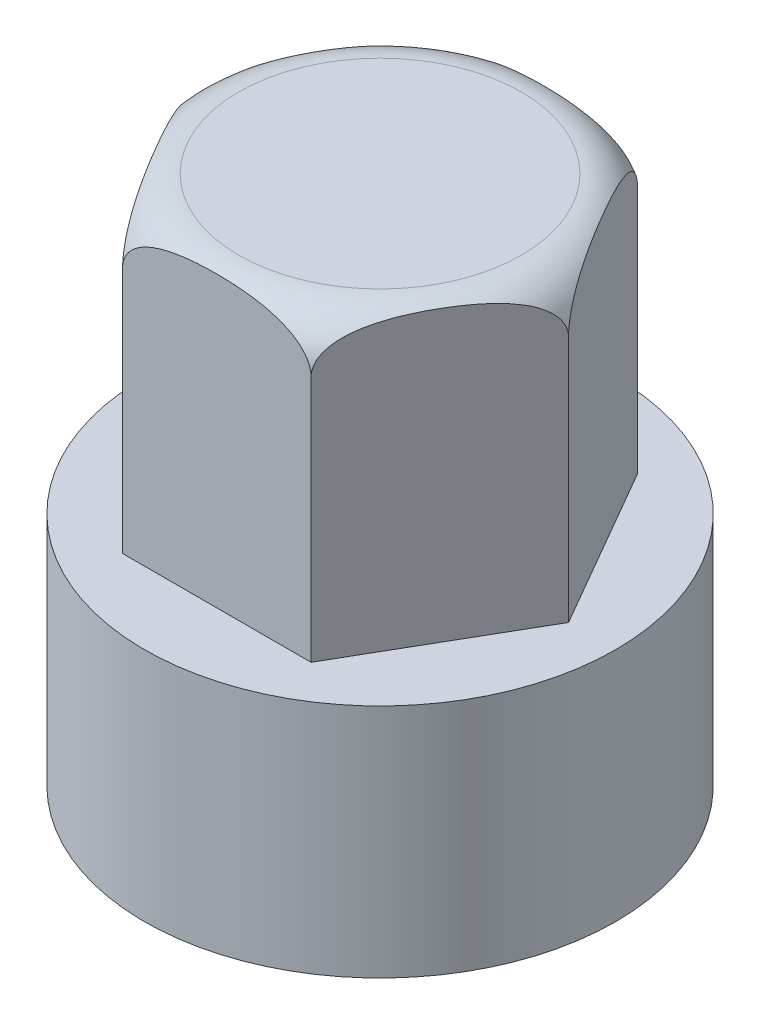
from build123d import *

# Parameters (mm, degrees)
HEX_32AF_SKETCH_OUTSIDE_W = 56.456
HEX_32AF_SKETCH_OUTSIDE_H = 56.456
HEX_32AF_CUT_DEPTH        = 25


with BuildPart() as part:
    # Cap Profile Sketch → Cap Body Revolve (revolve)
    with BuildSketch(Plane.XY):
        with BuildLine():
            Line((0, 0), (20, 0))
            Line((20, 0), (20, 20))
            Line((20, 20), (16, 20))
            Line((16, 20), (16, 41))
            ThreePointArc((16, 41), (14.828427125, 43.828427125), (12, 45))
            Line((12, 45), (0, 45))
            Line((0, 45), (0, 0))
        make_face()
    revolve(axis=Axis((0, 0, 0), (0, 1, 0)))

    # Hex 32AF Sketch outside → Hex 32AF Cut (cut)
    with BuildSketch(Plane(origin=(0, 45, 0), x_dir=(1, 0, 0), z_dir=(0, 1, 0))):
        Rectangle(HEX_32AF_SKETCH_OUTSIDE_W, HEX_32AF_SKETCH_OUTSIDE_H)
        Polygon((8, 13.856406461), (-8, 13.856406461), (-16, 0), (-8, -13.856406461), (8, -13.856406461), (16, 0), align=None, mode=Mode.SUBTRACT)
    extrude(amount=-HEX_32AF_CUT_DEPTH, mode=Mode.SUBTRACT)

    # Hex Chamfer 30deg Sketch → Hex Top Chamfer 30deg (revolve, cut)
    with BuildSketch(Plane.XY, mode=Mode.PRIVATE) as hex_top_chamfer_30deg_sk:
        with BuildLine():
            Line((0, 0), (12, 0))
            Line((12, 0), (12, 12))
            Line((12, 12), (9, 13.732050808))
            Line((9, 13.732050808), (9, 39))
            ThreePointArc((9, 39), (8.414213562, 40.414213562), (7, 41))
            Line((7, 41), (0, 41))
            Line((0, 41), (0, 0))
        make_face()
    revolve(hex_top_chamfer_30deg_sk.sketch.rotate(Axis((0, 0, 0), (0, 1, 0)), 90), axis=Axis((0, 0, 0), (0, 1, 0)), mode=Mode.SUBTRACT)


solid = part.part
